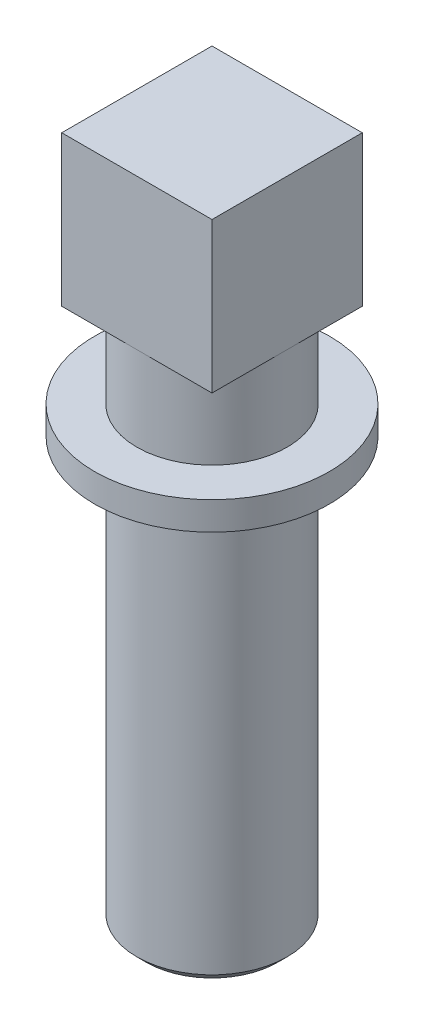
ISO-10303-21;
HEADER;
FILE_DESCRIPTION(('STEP AP214'),'2;1');
FILE_NAME('part.step','',(''),(''),'','','');
FILE_SCHEMA(('AUTOMOTIVE_DESIGN { 1 0 10303 214 1 1 1 1 }'));
ENDSEC;
DATA;
#1=APPLICATION_CONTEXT('core data for automotive mechanical design processes');
#2=APPLICATION_PROTOCOL_DEFINITION('international standard','automotive_design',2000,#1);
#3=PRODUCT_CONTEXT('',#1,'mechanical');
#4=PRODUCT('Part','Part','',(#3));
#5=PRODUCT_RELATED_PRODUCT_CATEGORY('part','',(#4));
#6=PRODUCT_DEFINITION_FORMATION('','',#4);
#7=PRODUCT_DEFINITION_CONTEXT('part definition',#1,'design');
#8=PRODUCT_DEFINITION('design','',#6,#7);
#9=PRODUCT_DEFINITION_SHAPE('','',#8);
#10=(LENGTH_UNIT() NAMED_UNIT(*) SI_UNIT(.MILLI.,.METRE.));
#11=(NAMED_UNIT(*) PLANE_ANGLE_UNIT() SI_UNIT($,.RADIAN.));
#12=(NAMED_UNIT(*) SI_UNIT($,.STERADIAN.) SOLID_ANGLE_UNIT());
#13=UNCERTAINTY_MEASURE_WITH_UNIT(LENGTH_MEASURE(1.E-05),#10,'distance_accuracy_value','');
#14=(GEOMETRIC_REPRESENTATION_CONTEXT(3) GLOBAL_UNCERTAINTY_ASSIGNED_CONTEXT((#13)) GLOBAL_UNIT_ASSIGNED_CONTEXT((#10,
#11,#12)) REPRESENTATION_CONTEXT('',''));
#15=CARTESIAN_POINT('',(0.,0.,0.));
#16=DIRECTION('',(0.,0.,1.));
#17=DIRECTION('',(1.,0.,0.));
#18=AXIS2_PLACEMENT_3D('',#15,#16,#17);
#19=CARTESIAN_POINT('',(0.,45.,0.));
#20=DIRECTION('',(0.,-1.,0.));
#21=DIRECTION('',(0.,0.,-1.));
#22=AXIS2_PLACEMENT_3D('',#19,#20,#21);
#23=CYLINDRICAL_SURFACE('',#22,8.);
#24=CARTESIAN_POINT('',(0.,1.00000000000004,0.));
#25=DIRECTION('',(0.,1.,0.));
#26=DIRECTION('',(0.,0.,1.));
#27=AXIS2_PLACEMENT_3D('',#24,#25,#26);
#28=CIRCLE('',#27,8.);
#29=CARTESIAN_POINT('',(0.,1.00000000000004,-8.));
#30=VERTEX_POINT('',#29);
#31=EDGE_CURVE('E140',#30,#30,#28,.T.);
#32=CARTESIAN_POINT('',(0.,45.,0.));
#33=DIRECTION('',(0.,1.,0.));
#34=DIRECTION('',(0.,0.,1.));
#35=AXIS2_PLACEMENT_3D('',#32,#33,#34);
#36=CIRCLE('',#35,8.);
#37=CARTESIAN_POINT('',(0.,45.,-8.));
#38=VERTEX_POINT('',#37);
#39=EDGE_CURVE('E135',#38,#38,#36,.T.);
#40=CARTESIAN_POINT('',(0.,1.00000000000004,-8.));
#41=CARTESIAN_POINT('',(0.,1.45833333333337,-8.));
#42=CARTESIAN_POINT('',(0.,1.9166666666667,-8.));
#43=CARTESIAN_POINT('',(0.,2.83333333333337,-8.));
#44=CARTESIAN_POINT('',(0.,3.2916666666667,-8.));
#45=CARTESIAN_POINT('',(0.,4.20833333333337,-8.));
#46=CARTESIAN_POINT('',(0.,4.6666666666667,-8.));
#47=CARTESIAN_POINT('',(0.,5.58333333333337,-8.));
#48=CARTESIAN_POINT('',(0.,6.0416666666667,-8.));
#49=CARTESIAN_POINT('',(0.,6.95833333333337,-8.));
#50=CARTESIAN_POINT('',(0.,7.4166666666667,-8.));
#51=CARTESIAN_POINT('',(0.,8.33333333333336,-8.));
#52=CARTESIAN_POINT('',(0.,8.7916666666667,-8.));
#53=CARTESIAN_POINT('',(0.,9.70833333333336,-8.));
#54=CARTESIAN_POINT('',(0.,10.1666666666667,-8.));
#55=CARTESIAN_POINT('',(0.,11.0833333333334,-8.));
#56=CARTESIAN_POINT('',(0.,11.5416666666667,-8.));
#57=CARTESIAN_POINT('',(0.,12.4583333333334,-8.));
#58=CARTESIAN_POINT('',(0.,12.9166666666667,-8.));
#59=CARTESIAN_POINT('',(0.,13.8333333333334,-8.));
#60=CARTESIAN_POINT('',(0.,14.2916666666667,-8.));
#61=CARTESIAN_POINT('',(0.,15.2083333333334,-8.));
#62=CARTESIAN_POINT('',(0.,15.6666666666667,-8.));
#63=CARTESIAN_POINT('',(0.,16.5833333333334,-8.));
#64=CARTESIAN_POINT('',(0.,17.0416666666667,-8.));
#65=CARTESIAN_POINT('',(0.,17.9583333333334,-8.));
#66=CARTESIAN_POINT('',(0.,18.4166666666667,-8.));
#67=CARTESIAN_POINT('',(0.,19.3333333333333,-8.));
#68=CARTESIAN_POINT('',(0.,19.7916666666667,-8.));
#69=CARTESIAN_POINT('',(0.,20.7083333333334,-8.));
#70=CARTESIAN_POINT('',(0.,21.1666666666667,-8.));
#71=CARTESIAN_POINT('',(0.,22.0833333333333,-8.));
#72=CARTESIAN_POINT('',(0.,22.5416666666667,-8.));
#73=CARTESIAN_POINT('',(0.,23.4583333333333,-8.));
#74=CARTESIAN_POINT('',(0.,23.9166666666667,-8.));
#75=CARTESIAN_POINT('',(0.,24.8333333333333,-8.));
#76=CARTESIAN_POINT('',(0.,25.2916666666667,-8.));
#77=CARTESIAN_POINT('',(0.,26.2083333333333,-8.));
#78=CARTESIAN_POINT('',(0.,26.6666666666667,-8.));
#79=CARTESIAN_POINT('',(0.,27.5833333333333,-8.));
#80=CARTESIAN_POINT('',(0.,28.0416666666667,-8.));
#81=CARTESIAN_POINT('',(0.,28.9583333333333,-8.));
#82=CARTESIAN_POINT('',(0.,29.4166666666667,-8.));
#83=CARTESIAN_POINT('',(0.,30.3333333333333,-8.));
#84=CARTESIAN_POINT('',(0.,30.7916666666667,-8.));
#85=CARTESIAN_POINT('',(0.,31.7083333333333,-8.));
#86=CARTESIAN_POINT('',(0.,32.1666666666667,-8.));
#87=CARTESIAN_POINT('',(0.,33.0833333333333,-8.));
#88=CARTESIAN_POINT('',(0.,33.5416666666667,-8.));
#89=CARTESIAN_POINT('',(0.,34.4583333333333,-8.));
#90=CARTESIAN_POINT('',(0.,34.9166666666667,-8.));
#91=CARTESIAN_POINT('',(0.,35.8333333333333,-8.));
#92=CARTESIAN_POINT('',(0.,36.2916666666667,-8.));
#93=CARTESIAN_POINT('',(0.,37.2083333333333,-8.));
#94=CARTESIAN_POINT('',(0.,37.6666666666667,-8.));
#95=CARTESIAN_POINT('',(0.,38.5833333333333,-8.));
#96=CARTESIAN_POINT('',(0.,39.0416666666667,-8.));
#97=CARTESIAN_POINT('',(0.,39.9583333333333,-8.));
#98=CARTESIAN_POINT('',(0.,40.4166666666667,-8.));
#99=CARTESIAN_POINT('',(0.,41.3333333333333,-8.));
#100=CARTESIAN_POINT('',(0.,41.7916666666667,-8.));
#101=CARTESIAN_POINT('',(0.,42.7083333333333,-8.));
#102=CARTESIAN_POINT('',(0.,43.1666666666667,-8.));
#103=CARTESIAN_POINT('',(0.,44.0833333333333,-8.));
#104=CARTESIAN_POINT('',(0.,44.5416666666667,-8.));
#105=CARTESIAN_POINT('',(0.,45.,-8.));
#106=B_SPLINE_CURVE_WITH_KNOTS('',3,(#40,#41,#42,#43,#44,#45,#46,#47,#48,#49,#50,#51,#52,#53,
#54,#55,#56,#57,#58,#59,#60,#61,#62,#63,#64,#65,#66,#67,#68,#69,#70,#71,#72,#73,#74,#75,#76,#77,
#78,#79,#80,#81,#82,#83,#84,#85,#86,#87,#88,#89,#90,#91,#92,#93,#94,#95,#96,#97,#98,#99,#100,
#101,#102,#103,#104,#105),.UNSPECIFIED.,.F.,.F.,(4,2,2,2,2,2,2,2,2,2,2,2,2,2,2,2,2,2,2,2,2,2,2,
2,2,2,2,2,2,2,2,2,4),(0.,1.375,2.75,4.125,5.5,6.87499999999999,8.24999999999999,
9.62499999999999,11.,12.375,13.75,15.125,16.5,17.875,19.25,20.625,22.,23.375,24.75,26.125,27.5,
28.875,30.25,31.625,33.,34.375,35.75,37.125,38.5,39.875,41.25,42.625,44.),.UNSPECIFIED.);
#107=EDGE_CURVE('BSEAM41',#30,#38,#106,.T.);
#108=ORIENTED_EDGE('',*,*,#31,.T.);
#109=ORIENTED_EDGE('',*,*,#39,.F.);
#110=ORIENTED_EDGE('',*,*,#107,.T.);
#111=ORIENTED_EDGE('',*,*,#107,.F.);
#112=EDGE_LOOP('',(#108,#110,#109,#111));
#113=FACE_BOUND('',#112,.T.);
#114=ADVANCED_FACE('F41',(#113),#23,.T.);
#115=CARTESIAN_POINT('',(0.,0.,0.));
#116=DIRECTION('',(0.,1.,0.));
#117=DIRECTION('',(0.,0.,1.));
#118=AXIS2_PLACEMENT_3D('',#115,#116,#117);
#119=PLANE('',#118);
#120=CARTESIAN_POINT('',(0.,0.,0.));
#121=DIRECTION('',(0.,1.,0.));
#122=DIRECTION('',(0.,0.,1.));
#123=AXIS2_PLACEMENT_3D('',#120,#121,#122);
#124=CIRCLE('',#123,6.99999999999996);
#125=CARTESIAN_POINT('',(0.,0.,6.99999999999996));
#126=VERTEX_POINT('',#125);
#127=EDGE_CURVE('E46',#126,#126,#124,.F.);
#128=ORIENTED_EDGE('',*,*,#127,.T.);
#129=EDGE_LOOP('',(#128));
#130=FACE_BOUND('',#129,.T.);
#131=ADVANCED_FACE('F143',(#130),#119,.F.);
#132=CARTESIAN_POINT('',(0.,1.00000000000004,0.));
#133=DIRECTION('',(0.,1.,0.));
#134=DIRECTION('',(0.,0.,1.));
#135=AXIS2_PLACEMENT_3D('',#132,#133,#134);
#136=CONICAL_SURFACE('',#135,8.,0.785398163397449);
#137=ORIENTED_EDGE('',*,*,#127,.F.);
#138=EDGE_LOOP('',(#137));
#139=FACE_BOUND('',#138,.T.);
#140=ORIENTED_EDGE('',*,*,#31,.F.);
#141=EDGE_LOOP('',(#140));
#142=FACE_BOUND('',#141,.T.);
#143=ADVANCED_FACE('F42',(#139,#142),#136,.T.);
#144=CARTESIAN_POINT('',(0.,48.,0.));
#145=DIRECTION('',(0.,-1.,0.));
#146=DIRECTION('',(0.,0.,-1.));
#147=AXIS2_PLACEMENT_3D('',#144,#145,#146);
#148=CYLINDRICAL_SURFACE('',#147,12.5);
#149=CARTESIAN_POINT('',(0.,48.,0.));
#150=DIRECTION('',(0.,1.,0.));
#151=DIRECTION('',(0.,0.,1.));
#152=AXIS2_PLACEMENT_3D('',#149,#150,#151);
#153=CIRCLE('',#152,12.5);
#154=CARTESIAN_POINT('',(0.,48.,12.5));
#155=VERTEX_POINT('',#154);
#156=EDGE_CURVE('E133',#155,#155,#153,.T.);
#157=ORIENTED_EDGE('',*,*,#156,.F.);
#158=EDGE_LOOP('',(#157));
#159=FACE_BOUND('',#158,.T.);
#160=CARTESIAN_POINT('',(0.,45.,0.));
#161=DIRECTION('',(0.,1.,0.));
#162=DIRECTION('',(0.,0.,1.));
#163=AXIS2_PLACEMENT_3D('',#160,#161,#162);
#164=CIRCLE('',#163,12.5);
#165=CARTESIAN_POINT('',(0.,45.,12.5));
#166=VERTEX_POINT('',#165);
#167=EDGE_CURVE('E129',#166,#166,#164,.T.);
#168=ORIENTED_EDGE('',*,*,#167,.T.);
#169=EDGE_LOOP('',(#168));
#170=FACE_BOUND('',#169,.T.);
#171=ADVANCED_FACE('F146',(#159,#170),#148,.T.);
#172=CARTESIAN_POINT('',(0.,48.,0.));
#173=DIRECTION('',(0.,1.,0.));
#174=DIRECTION('',(0.,0.,1.));
#175=AXIS2_PLACEMENT_3D('',#172,#173,#174);
#176=PLANE('',#175);
#177=CARTESIAN_POINT('',(0.,48.,0.));
#178=DIRECTION('',(0.,1.,0.));
#179=DIRECTION('',(0.,0.,1.));
#180=AXIS2_PLACEMENT_3D('',#177,#178,#179);
#181=CIRCLE('',#180,8.);
#182=CARTESIAN_POINT('',(0.,48.,8.));
#183=VERTEX_POINT('',#182);
#184=EDGE_CURVE('E11',#183,#183,#181,.T.);
#185=ORIENTED_EDGE('',*,*,#184,.F.);
#186=EDGE_LOOP('',(#185));
#187=FACE_BOUND('',#186,.T.);
#188=ORIENTED_EDGE('',*,*,#156,.T.);
#189=EDGE_LOOP('',(#188));
#190=FACE_BOUND('',#189,.T.);
#191=ADVANCED_FACE('F155',(#187,#190),#176,.T.);
#192=CARTESIAN_POINT('',(0.,45.,0.));
#193=DIRECTION('',(0.,1.,0.));
#194=DIRECTION('',(0.,0.,1.));
#195=AXIS2_PLACEMENT_3D('',#192,#193,#194);
#196=PLANE('',#195);
#197=ORIENTED_EDGE('',*,*,#39,.T.);
#198=EDGE_LOOP('',(#197));
#199=FACE_BOUND('',#198,.T.);
#200=ORIENTED_EDGE('',*,*,#167,.F.);
#201=EDGE_LOOP('',(#200));
#202=FACE_BOUND('',#201,.T.);
#203=ADVANCED_FACE('F161',(#199,#202),#196,.F.);
#204=CARTESIAN_POINT('',(0.,57.,0.));
#205=DIRECTION('',(0.,-1.,0.));
#206=DIRECTION('',(0.,0.,-1.));
#207=AXIS2_PLACEMENT_3D('',#204,#205,#206);
#208=CYLINDRICAL_SURFACE('',#207,8.);
#209=CARTESIAN_POINT('',(0.,57.,0.));
#210=DIRECTION('',(0.,1.,0.));
#211=DIRECTION('',(0.,0.,1.));
#212=AXIS2_PLACEMENT_3D('',#209,#210,#211);
#213=CIRCLE('',#212,8.);
#214=CARTESIAN_POINT('',(0.,57.,8.));
#215=VERTEX_POINT('',#214);
#216=CARTESIAN_POINT('',(8.,57.,0.));
#217=VERTEX_POINT('',#216);
#218=EDGE_CURVE('E124',#215,#217,#213,.T.);
#219=ORIENTED_EDGE('',*,*,#218,.F.);
#220=CARTESIAN_POINT('',(-8.,57.,0.));
#221=VERTEX_POINT('',#220);
#222=EDGE_CURVE('E59',#221,#215,#213,.T.);
#223=ORIENTED_EDGE('',*,*,#222,.F.);
#224=CARTESIAN_POINT('',(0.,57.,-8.));
#225=VERTEX_POINT('',#224);
#226=EDGE_CURVE('E65',#225,#221,#213,.T.);
#227=ORIENTED_EDGE('',*,*,#226,.F.);
#228=EDGE_CURVE('E126',#217,#225,#213,.T.);
#229=ORIENTED_EDGE('',*,*,#228,.F.);
#230=EDGE_LOOP('',(#219,#223,#227,#229));
#231=FACE_BOUND('',#230,.T.);
#232=ORIENTED_EDGE('',*,*,#184,.T.);
#233=EDGE_LOOP('',(#232));
#234=FACE_BOUND('',#233,.T.);
#235=ADVANCED_FACE('F168',(#231,#234),#208,.T.);
#236=CARTESIAN_POINT('',(0.,57.,0.));
#237=DIRECTION('',(0.,1.,0.));
#238=DIRECTION('',(0.,0.,1.));
#239=AXIS2_PLACEMENT_3D('',#236,#237,#238);
#240=PLANE('',#239);
#241=DIRECTION('',(1.,0.,0.));
#242=VECTOR('',#241,1.);
#243=CARTESIAN_POINT('',(-8.,57.,8.));
#244=LINE('',#243,#242);
#245=CARTESIAN_POINT('',(8.,57.,8.));
#246=VERTEX_POINT('',#245);
#247=EDGE_CURVE('E310',#215,#246,#244,.T.);
#248=ORIENTED_EDGE('',*,*,#247,.F.);
#249=ORIENTED_EDGE('',*,*,#218,.T.);
#250=DIRECTION('',(0.,0.,-1.));
#251=VECTOR('',#250,1.);
#252=CARTESIAN_POINT('',(8.,57.,-8.));
#253=LINE('',#252,#251);
#254=EDGE_CURVE('E291',#246,#217,#253,.T.);
#255=ORIENTED_EDGE('',*,*,#254,.F.);
#256=EDGE_LOOP('',(#248,#249,#255));
#257=FACE_BOUND('',#256,.T.);
#258=ADVANCED_FACE('F173',(#257),#240,.F.);
#259=CARTESIAN_POINT('',(8.,57.,-8.));
#260=VERTEX_POINT('',#259);
#261=EDGE_CURVE('E118',#217,#260,#253,.T.);
#262=ORIENTED_EDGE('',*,*,#261,.F.);
#263=ORIENTED_EDGE('',*,*,#228,.T.);
#264=DIRECTION('',(-1.,0.,0.));
#265=VECTOR('',#264,1.);
#266=CARTESIAN_POINT('',(-8.,57.,-8.));
#267=LINE('',#266,#265);
#268=EDGE_CURVE('E292',#260,#225,#267,.T.);
#269=ORIENTED_EDGE('',*,*,#268,.F.);
#270=EDGE_LOOP('',(#262,#263,#269));
#271=FACE_BOUND('',#270,.T.);
#272=ADVANCED_FACE('F186',(#271),#240,.F.);
#273=CARTESIAN_POINT('',(-8.,57.,-8.));
#274=VERTEX_POINT('',#273);
#275=EDGE_CURVE('E296',#225,#274,#267,.T.);
#276=ORIENTED_EDGE('',*,*,#275,.F.);
#277=ORIENTED_EDGE('',*,*,#226,.T.);
#278=DIRECTION('',(0.,0.,1.));
#279=VECTOR('',#278,1.);
#280=CARTESIAN_POINT('',(-8.,57.,-8.));
#281=LINE('',#280,#279);
#282=EDGE_CURVE('E302',#274,#221,#281,.T.);
#283=ORIENTED_EDGE('',*,*,#282,.F.);
#284=EDGE_LOOP('',(#276,#277,#283));
#285=FACE_BOUND('',#284,.T.);
#286=ADVANCED_FACE('F222',(#285),#240,.F.);
#287=CARTESIAN_POINT('',(-8.,57.,8.));
#288=VERTEX_POINT('',#287);
#289=EDGE_CURVE('E303',#221,#288,#281,.T.);
#290=ORIENTED_EDGE('',*,*,#289,.F.);
#291=ORIENTED_EDGE('',*,*,#222,.T.);
#292=EDGE_CURVE('E112',#288,#215,#244,.T.);
#293=ORIENTED_EDGE('',*,*,#292,.F.);
#294=EDGE_LOOP('',(#290,#291,#293));
#295=FACE_BOUND('',#294,.T.);
#296=ADVANCED_FACE('F176',(#295),#240,.F.);
#297=CARTESIAN_POINT('',(8.,73.,-8.));
#298=DIRECTION('',(-1.,0.,0.));
#299=DIRECTION('',(0.,0.,1.));
#300=AXIS2_PLACEMENT_3D('',#297,#298,#299);
#301=PLANE('',#300);
#302=ORIENTED_EDGE('',*,*,#254,.T.);
#303=ORIENTED_EDGE('',*,*,#261,.T.);
#304=DIRECTION('',(0.,-1.,0.));
#305=VECTOR('',#304,1.);
#306=CARTESIAN_POINT('',(8.,73.,-8.));
#307=LINE('',#306,#305);
#308=CARTESIAN_POINT('',(8.,73.,-8.));
#309=VERTEX_POINT('',#308);
#310=EDGE_CURVE('E100',#309,#260,#307,.T.);
#311=ORIENTED_EDGE('',*,*,#310,.F.);
#312=DIRECTION('',(0.,0.,-1.));
#313=VECTOR('',#312,1.);
#314=CARTESIAN_POINT('',(8.,73.,-8.));
#315=LINE('',#314,#313);
#316=CARTESIAN_POINT('',(8.,73.,8.));
#317=VERTEX_POINT('',#316);
#318=EDGE_CURVE('E102',#317,#309,#315,.T.);
#319=ORIENTED_EDGE('',*,*,#318,.F.);
#320=DIRECTION('',(0.,-1.,0.));
#321=VECTOR('',#320,1.);
#322=CARTESIAN_POINT('',(8.,73.,8.));
#323=LINE('',#322,#321);
#324=EDGE_CURVE('E298',#317,#246,#323,.T.);
#325=ORIENTED_EDGE('',*,*,#324,.T.);
#326=EDGE_LOOP('',(#302,#303,#311,#319,#325));
#327=FACE_BOUND('',#326,.T.);
#328=ADVANCED_FACE('F120',(#327),#301,.F.);
#329=CARTESIAN_POINT('',(-8.,73.,-8.));
#330=DIRECTION('',(0.,0.,1.));
#331=DIRECTION('',(1.,0.,0.));
#332=AXIS2_PLACEMENT_3D('',#329,#330,#331);
#333=PLANE('',#332);
#334=ORIENTED_EDGE('',*,*,#268,.T.);
#335=ORIENTED_EDGE('',*,*,#275,.T.);
#336=DIRECTION('',(0.,-1.,0.));
#337=VECTOR('',#336,1.);
#338=CARTESIAN_POINT('',(-8.,73.,-8.));
#339=LINE('',#338,#337);
#340=CARTESIAN_POINT('',(-8.,73.,-8.));
#341=VERTEX_POINT('',#340);
#342=EDGE_CURVE('E103',#341,#274,#339,.T.);
#343=ORIENTED_EDGE('',*,*,#342,.F.);
#344=DIRECTION('',(-1.,0.,0.));
#345=VECTOR('',#344,1.);
#346=CARTESIAN_POINT('',(-8.,73.,-8.));
#347=LINE('',#346,#345);
#348=EDGE_CURVE('E91',#309,#341,#347,.T.);
#349=ORIENTED_EDGE('',*,*,#348,.F.);
#350=ORIENTED_EDGE('',*,*,#310,.T.);
#351=EDGE_LOOP('',(#334,#335,#343,#349,#350));
#352=FACE_BOUND('',#351,.T.);
#353=ADVANCED_FACE('F97',(#352),#333,.F.);
#354=CARTESIAN_POINT('',(-8.,73.,-8.));
#355=DIRECTION('',(1.,0.,0.));
#356=DIRECTION('',(0.,0.,-1.));
#357=AXIS2_PLACEMENT_3D('',#354,#355,#356);
#358=PLANE('',#357);
#359=ORIENTED_EDGE('',*,*,#282,.T.);
#360=ORIENTED_EDGE('',*,*,#289,.T.);
#361=DIRECTION('',(0.,-1.,0.));
#362=VECTOR('',#361,1.);
#363=CARTESIAN_POINT('',(-8.,73.,8.));
#364=LINE('',#363,#362);
#365=CARTESIAN_POINT('',(-8.,73.,8.));
#366=VERTEX_POINT('',#365);
#367=EDGE_CURVE('E121',#366,#288,#364,.T.);
#368=ORIENTED_EDGE('',*,*,#367,.F.);
#369=DIRECTION('',(0.,0.,1.));
#370=VECTOR('',#369,1.);
#371=CARTESIAN_POINT('',(-8.,73.,-8.));
#372=LINE('',#371,#370);
#373=EDGE_CURVE('E104',#341,#366,#372,.T.);
#374=ORIENTED_EDGE('',*,*,#373,.F.);
#375=ORIENTED_EDGE('',*,*,#342,.T.);
#376=EDGE_LOOP('',(#359,#360,#368,#374,#375));
#377=FACE_BOUND('',#376,.T.);
#378=ADVANCED_FACE('F177',(#377),#358,.F.);
#379=CARTESIAN_POINT('',(-8.,73.,8.));
#380=DIRECTION('',(0.,0.,-1.));
#381=DIRECTION('',(-1.,0.,0.));
#382=AXIS2_PLACEMENT_3D('',#379,#380,#381);
#383=PLANE('',#382);
#384=ORIENTED_EDGE('',*,*,#292,.T.);
#385=ORIENTED_EDGE('',*,*,#247,.T.);
#386=ORIENTED_EDGE('',*,*,#324,.F.);
#387=DIRECTION('',(1.,0.,0.));
#388=VECTOR('',#387,1.);
#389=CARTESIAN_POINT('',(-8.,73.,8.));
#390=LINE('',#389,#388);
#391=EDGE_CURVE('E109',#366,#317,#390,.T.);
#392=ORIENTED_EDGE('',*,*,#391,.F.);
#393=ORIENTED_EDGE('',*,*,#367,.T.);
#394=EDGE_LOOP('',(#384,#385,#386,#392,#393));
#395=FACE_BOUND('',#394,.T.);
#396=ADVANCED_FACE('F185',(#395),#383,.F.);
#397=CARTESIAN_POINT('',(0.,73.,0.));
#398=DIRECTION('',(0.,1.,0.));
#399=DIRECTION('',(0.,0.,1.));
#400=AXIS2_PLACEMENT_3D('',#397,#398,#399);
#401=PLANE('',#400);
#402=ORIENTED_EDGE('',*,*,#318,.T.);
#403=ORIENTED_EDGE('',*,*,#348,.T.);
#404=ORIENTED_EDGE('',*,*,#373,.T.);
#405=ORIENTED_EDGE('',*,*,#391,.T.);
#406=EDGE_LOOP('',(#402,#403,#404,#405));
#407=FACE_BOUND('',#406,.T.);
#408=ADVANCED_FACE('F108',(#407),#401,.T.);
#409=CLOSED_SHELL('',(#114,#131,#143,#171,#191,#203,#235,#258,#272,#286,#296,#328,#353,#378,
#396,#408));
#410=MANIFOLD_SOLID_BREP('B2',#409);
#411=ADVANCED_BREP_SHAPE_REPRESENTATION('',(#18,#410),#14);
#412=SHAPE_DEFINITION_REPRESENTATION(#9,#411);
ENDSEC;
END-ISO-10303-21;
